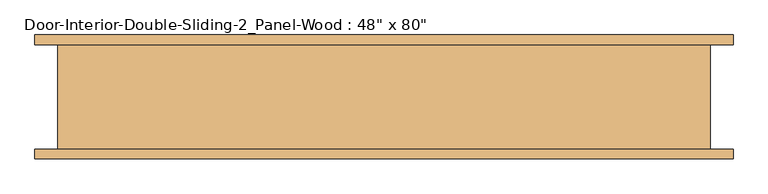
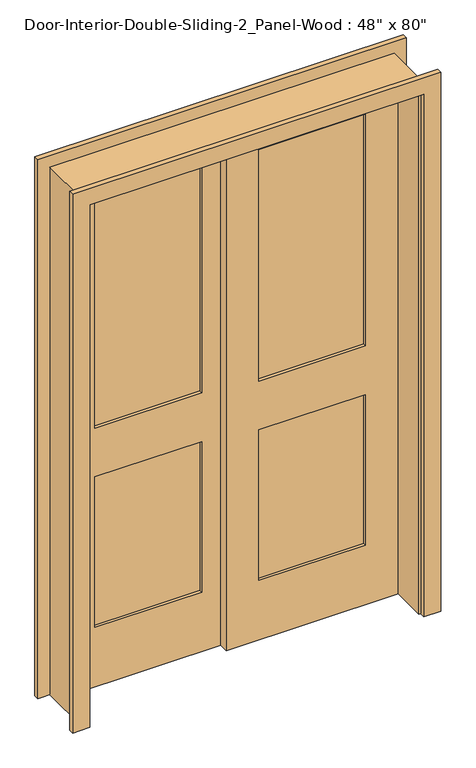
"""IFC4 building model written with IfcOpenShell, lengths in millimetres: door geometry."""

from ifc_helpers import new_model, si_unit, frame, origin, place, context, project, spatial, polyline, outline, extrude, source, transform, mapped, element, save


def door_f9cb40a9(model_context):
    return source(origin(), model_context, "Body", "SweptSolid", [
        extrude(outline(polyline([(488.95, 40.2166667), (95.25, 40.2166667), (95.25, 51.8583333), (488.95, 51.8583333), (488.95, 40.2166667)])), frame((0.0, 0.0, 1009.65), z_axis=(0.0, 0.0, 1.0), x_axis=(1.0, 0.0, 0.0)), (0.0, 0.0, 1.0), 903.2875),
        extrude(outline(polyline([(488.95, 40.2166667), (95.25, 40.2166667), (95.25, 51.8583333), (488.95, 51.8583333), (488.95, 40.2166667)])), frame((0.0, 0.0, 231.775), z_axis=(0.0, 0.0, 1.0), x_axis=(1.0, 0.0, 0.0)), (0.0, 0.0, 1.0), 587.375),
        extrude(outline(polyline([(2032.0, -25.4), (0.0, -25.4), (0.0, 609.6), (2032.0, 609.6), (2032.0, -25.4)]), holes=[polyline([(1912.9375, 95.25), (1912.9375, 488.95), (1009.65, 488.95), (1009.65, 95.25), (1912.9375, 95.25)]), polyline([(819.15, 95.25), (819.15, 488.95), (231.775, 488.95), (231.775, 95.25), (819.15, 95.25)])]), frame((0.0, 28.575, 0.0), z_axis=(0.0, 1.0, 0.0), x_axis=(0.0, 0.0, 1.0)), (0.0, 0.0, 1.0), 34.925),
        extrude(outline(polyline([(-95.25, 75.1416667), (-488.95, 75.1416667), (-488.95, 86.7833333), (-95.25, 86.7833333), (-95.25, 75.1416667)])), frame((0.0, 0.0, 1009.65), z_axis=(0.0, 0.0, 1.0), x_axis=(1.0, 0.0, 0.0)), (0.0, 0.0, 1.0), 903.2875),
        extrude(outline(polyline([(-95.25, 75.1416667), (-488.95, 75.1416667), (-488.95, 86.7833333), (-95.25, 86.7833333), (-95.25, 75.1416667)])), frame((0.0, 0.0, 231.775), z_axis=(0.0, 0.0, 1.0), x_axis=(1.0, 0.0, 0.0)), (0.0, 0.0, 1.0), 587.375),
        extrude(outline(polyline([(2032.0, -609.6), (0.0, -609.6), (0.0, 25.4), (2032.0, 25.4), (2032.0, -609.6)]), holes=[polyline([(1912.9375, -488.95), (1912.9375, -95.25), (1009.65, -95.25), (1009.65, -488.95), (1912.9375, -488.95)]), polyline([(819.15, -488.95), (819.15, -95.25), (231.775, -95.25), (231.775, -488.95), (819.15, -488.95)])]), frame((0.0, 63.5, 0.0), z_axis=(0.0, 1.0, 0.0), x_axis=(0.0, 0.0, 1.0)), (0.0, 0.0, 1.0), 34.925),
        extrude(outline(polyline([(0.0, 609.6), (0.0, 635.0), (2057.4, 635.0), (2057.4, -635.0), (0.0, -635.0), (0.0, -609.6), (2032.0, -609.6), (2032.0, 609.6), (0.0, 609.6)])), frame((0.0, -104.775, 0.0), z_axis=(0.0, 1.0, 0.0), x_axis=(0.0, 0.0, 1.0)), (0.0, 0.0, 1.0), 203.2),
        extrude(outline(polyline([(0.0, 615.95), (0.0, 679.45), (2101.85, 679.45), (2101.85, -679.45), (0.0, -679.45), (0.0, -615.95), (2038.35, -615.95), (2038.35, 615.95), (0.0, 615.95)])), frame((0.0, -123.825, 0.0), z_axis=(0.0, 1.0, 0.0), x_axis=(0.0, 0.0, 1.0)), (0.0, 0.0, 1.0), 19.05),
        extrude(outline(polyline([(0.0, 615.95), (0.0, 679.45), (2101.85, 679.45), (2101.85, -679.45), (0.0, -679.45), (0.0, -615.95), (2038.35, -615.95), (2038.35, 615.95), (0.0, 615.95)])), frame((0.0, 98.425, 0.0), z_axis=(0.0, 1.0, 0.0), x_axis=(0.0, 0.0, 1.0)), (0.0, 0.0, 1.0), 19.05),
    ])


if __name__ == "__main__":
    model = new_model("IFC4")
    model_context = context("Model", 3, world=origin())
    ifc_project = project(units=[si_unit("LENGTHUNIT", "METRE", prefix="MILLI")], contexts=[model_context])
    site = spatial("IfcSite", under=ifc_project)
    building = spatial("IfcBuilding", under=site)
    placement = place(None, origin())
    door_shape = door_f9cb40a9(model_context)
    element("IfcDoor", 1, ObjectType="Door-Interior-Double-Sliding-2_Panel-Wood : 48\" x 80\"", at=placement, inside=building, context=model_context, shape_type="MappedRepresentation", body=[
        mapped(door_shape, transform((0.0, 0.0, 0.0), x_axis=(1.0, 0.0, 0.0), y_axis=(0.0, 1.0, 0.0), z_axis=(0.0, 0.0, 1.0))),
    ])
    save(model, "model.ifc")

# Revit data of these elements
# Type "Door-Interior-Double-Sliding-2_Panel-Wood : 48\" x 80\""
#   Type Mark = "10"
#   Assembly Code = "C1020300"
#   Analytic Construction = "Wooden"
#   Top Rail = 0' - 4 11/16"
#   Thickness = 0' - 1 3/8"
#   Thermal Resistance (R) = 2.5876 (h·ft²·°F)/BTU
#   Stiles = 0' - 4 3/4"
#   Rough Width = 4' - 2"
#   Rough Height = 6' - 9"
#   Lock Rail = 0' - 7 1/2"
#   Height = 6' - 8"
#   Width = 4' - 0"
#   Heat Transfer Coefficient (U) = 0.3865 BTU/(h·ft²·°F)
#   Bottom Rail = 0' - 9 1/8"
#   Trim Material = Cherry
#   Panel Material = Cherry
#   Frame Material = Cherry
#   Visual Light Transmittance = 0
#   Solar Heat Gain Coefficient = 0
#   Wall Closure = (empty or 0)
#   Function = (empty or 0)
# Element 1 (IfcDoor, "Door-Interior-Double-Sliding-2_Panel-Wood : 48\" x 80\"")
#   Materials on its faces: "Cherry"
# Materials
#   "Cherry": class "Wood", colour RGB 226 177 128, transparency 0, Description = "Prunus Serotina", Cost = 0
